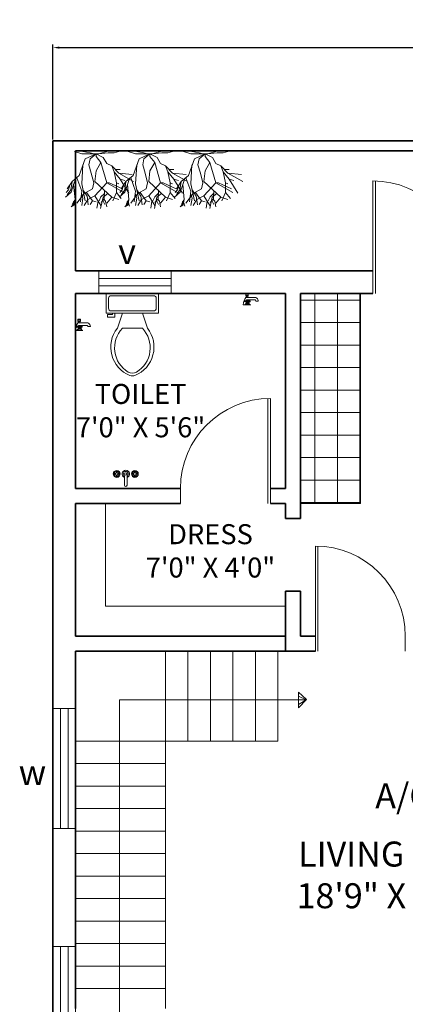
# Model space of a CAD drawing. Units: inches. Extents: x 2729 to 3178, y 5006 to 5809.
# Tile 3 of 4: x 2735 to 2889, y 5415 to 5809. Entities that reach past the tile are written whole.
import ezdxf

# ---------------------------------------------------------------- set-up
doc = ezdxf.new("R2010")
doc.units = ezdxf.units.IN
doc.layers.get('Defpoints').update_dxf_attribs({"color": 72})
for name, color, linetype, lineweight in [('A-ANNO-DIMS', 2, 'Continuous', 18), ('A-ANNO-TEXT', 7, 'Continuous', 18), ('A-AREA-IDEN', 7, 'Continuous', 25), ('A-DOOR', 4, 'Continuous', 18), ('A-FLOR-CASE', 8, 'Continuous', 18), ('A-FLOR-FIXT', 9, 'Continuous', 18), ('A-FLOR-PATT', 9, 'Continuous', 13), ('A-FLOR-STRS', 7, 'Continuous', 18), ('A-GLAZ', 4, 'Continuous', 18), ('A-WALL', 7, 'Continuous', 35), ('L-PLNT', 72, 'Continuous', 13)]:
    doc.layers.add(name, color=color, linetype=linetype, lineweight=lineweight)
doc.styles.get("Standard").update_dxf_attribs({"font": 'arial.ttf'})
doc.dimstyles.new('ISO-25', dxfattribs={"dimtxt": 2.5, "dimasz": 2.5, "dimexe": 1.25, "dimexo": 0.625, "dimtad": 1, "dimdec": 0, "dimlunit": 3, "dimtxsty": 'Standard', "dimcen": 2.5, "dimadec": 0, "dimazin": 0, "dimtfac": 1, "dimtdec": 0, "dimtmove": 0, "dimatfit": 3, "dimfxl": 1, "dimarcsym": 0})

# ---------------------------------------------------------------- blocks, each defined once
blk = doc.blocks.new('*D1')
at = {"layer": 'A-ANNO-DIMS', "color": 0, "lineweight": -2, "transparency": 16777216}
for p, q in [((2748.18, 5761.26), (2748.18, 5799.21)), ((2750.68, 5797.96), (3069.68, 5797.96)), ((3072.18, 5761.26), (3072.18, 5799.21))]:
    blk.add_line(p, q, dxfattribs=at)
at = {"layer": 'A-ANNO-DIMS', "color": 0, "transparency": 16777216}
for points in [[(2750.68, 5798.38), (2750.68, 5797.54), (2748.18, 5797.96)], [(3069.68, 5798.38), (3069.68, 5797.54), (3072.18, 5797.96)]]:
    blk.add_solid(points, dxfattribs=at)
at = {"layer": 'Defpoints', "color": 0, "transparency": 16777216}
for p in [(3072.18, 5797.96), (2748.18, 5760.64), (3072.18, 5760.64)]:
    blk.add_point(p, dxfattribs=at)
at = {"layer": 'A-ANNO-DIMS', "color": 0, "transparency": 16777216, "insert": (2910.18, 5803.61), "char_height": 2.5, "attachment_point": 5}
blk.add_mtext("{\\H4x;27'}", dxfattribs=at)
blk = doc.blocks.new('Faucet - Bathroom side')
for p, q in [((-0.625, 4.25), (0.375, 4.25)), ((-1.625, 0), (-1.375, 0)), ((-1.375, 0), (1.375, 0)), ((-0.88366, 0.25), (0.88424, 0.25)), ((0.375, 3.75), (-0.625, 3.75)), ((-0.625, 3), (3.375, 3)), ((-0.375, 1.625), (-0.625, 1.625)), ((-0.375, 1.375), (-0.625, 1.375)), ((0.48078, 0.75), (-0.47286, 0.75)), ((-0.375, 3), (-0.375, 3.5)), ((0.125, 3.5), (0.125, 3)), ((2.875, 2), (0.375, 2)), ((0.375, 1.625), (0.625, 1.625)), ((0.375, 1.375), (0.625, 1.375)), ((4.375, 1.5), (3.375, 1.5))]:
    blk.add_line(p, q)
for points in [[(-0.625, 3.75), (-0.625, 4.25)], [(-0.375, 4.5), (0.125, 4.5)], [(0.375, 4.25), (0.375, 3.75)], [(0.125, 3.5), (-0.375, 3.5)]]:
    blk.add_lwpolyline(points)
blk.add_lwpolyline([(-0.375, 1), (-0.375, 2), (0.375, 2), (0.375, 1)], close=True)
for centre in [(-0.875, 1.5), (0, 1.5), (0.875, 1.5)]:
    blk.add_circle(centre, 0.27951)
for centre, radius, start, end in [((-0.38253, 4.2575), 0.24259, 88.22243, 181.7776), ((0.13252, 4.2575), 0.24259, 358.2224, 91.77757), ((3.45929, -0.0281), 5.08436, 143.4467, 179.6834), ((-1.75, 1.375), 1.42522, 285.2551, 344.7449), ((-0.38253, 3.7424), 0.24259, 178.2224, 271.7776), ((0.13252, 3.7424), 0.24259, 268.2224, 1.777565), ((1.75, 1.375), 1.42522, 195.2551, 254.7449), ((-2.49562, -0.286), 3.38273, 9.709485, 29.48735), ((2.96867, 1.5936), 0.41699, 347.0192, 102.9808), ((2.70708, 1.4714), 1.66816, 0.9827695, 66.39737)]:
    blk.add_arc(centre, radius, start, end)
blk = doc.blocks.new('Toilet - top')
for p, q in [((9.5, -6), (9.5, -2)), ((-10, -8.5), (-8, -8.5)), ((-10, -9.5), (-10, -8.5)), ((-7, -9.5), (-10, -9.5)), ((-8, -8.5), (-8, -8)), ((-7, -8), (-7, -9.5)), ((-4, -8), (-6, -14)), ((4, -8), (6, -14)), ((4, -14), (-4, -14))]:
    blk.add_line(p, q)
blk.add_lwpolyline([(10.5, -8), (10.5, 0), (-10.5, 0), (-10.5, -8)], close=True)
for points in [[(-9.5, -2), (-9.5, -6)], [(8.5, -1), (-8.5, -1)], [(-8.5, -7), (8.5, -7)]]:
    blk.add_lwpolyline(points)
for centre, radius, start, end in [((-8.62, -1.88), 0.884, 81.8699, 188.1301), ((8.62, -1.88), 0.884, 351.8699, 98.1301), ((-8.62, -6.12), 0.884, 171.8699, 278.1301), ((8.62, -6.12), 0.884, 261.8699, 8.1301), ((3.52, -21.58), 12.17, 141.4691, 247.9714), ((4.2, -21.82), 11.33, 136.3677, 238.9468), ((-3.52, -21.58), 12.17, 292.0284, 38.5307), ((-4.2, -21.82), 11.33, 301.053, 43.6321), ((0, -27.88), 4, 245.7318, 294.2682), ((0, -29), 4, 254.8605, 285.1395)]:
    blk.add_arc(centre, radius, start, end)
blk = doc.blocks.new('Faucet - Bathroom top')
for p, q in [((-4.107, 0.125), (-4.375, 0.125)), ((-3.75, 0.4788), (-3.75, 0.75)), ((-3.5, 0.482), (-3.5, 0.75)), ((-3.1461, 0.125), (-2.875, 0.125)), ((3.143, 0.125), (2.875, 0.125)), ((3.5, 0.4788), (3.5, 0.75)), ((3.75, 0.482), (3.75, 0.75)), ((4.1039, 0.125), (4.375, 0.125)), ((-4.1039, -0.125), (-4.375, -0.125)), ((-3.75, -0.4821), (-3.75, -0.75)), ((-3.5, -0.4789), (-3.5, -0.75)), ((-3.143, -0.125), (-2.875, -0.125)), ((-0.5, -0.8639), (-0.5, -4.5)), ((0.5, -4.5), (0.5, -0.8631)), ((3.1461, -0.125), (2.875, -0.125)), ((3.5, -0.4821), (3.5, -0.75)), ((3.75, -0.4789), (3.75, -0.75)), ((4.107, -0.125), (4.375, -0.125))]:
    blk.add_line(p, q)
for centre, radius in [((-3.625, 0), 1.375), ((-4.625, 0), 0.2795), ((-3.625, 0), 0.5), ((-3.625, 1), 0.2795), ((-2.625, 0), 0.2795), ((0, 0), 0.5), ((3.625, 0), 1.375), ((2.625, 0), 0.2795), ((3.625, 0), 0.5), ((3.625, 1), 0.2795), ((4.625, 0), 0.2795), ((-3.625, -1), 0.2795), ((3.625, -1), 0.2795)]:
    blk.add_circle(centre, radius)
for centre, radius, start, end in [((-3.625, 0), 1, 105.2407, 164.2093), ((-3.625, 0), 1, 16.44125, 74.07887), ((0, 0), 1.5, 289.6514, 250.3603), ((0, 0), 1, 300.3431, 239.7554), ((3.625, 0), 1, 106.12, 164.0884), ((3.625, 0), 1, 16.23422, 73.90469), ((-3.625, 0), 1, 196.2342, 253.9047), ((-3.625, 0), 1, 286.12, 344.0884), ((3.625, 0), 1, 196.4413, 254.0789), ((3.625, 0), 1, 285.2407, 344.2093), ((0, -4.5), 0.5, 180, 0)]:
    blk.add_arc(centre, radius, start, end)
blk = doc.blocks.new('*U13')
for p, q in [((-377.952, 463.296), (-329.184, 524.256)), ((-316.7634, 502.285), (-327.6092, 559.9176)), ((-296.5958, 484.4034), (-316.7634, 502.285)), ((-286.512, 498.3226), (-307.4416, 538.0736)), ((-302.7934, 478.4344), (-270.256, 518.1854)), ((-290.3982, 464.5406), (-265.6078, 577.8246)), ((-268.7066, 458.5716), (-250.0884, 500.3038)), ((-207.264, 451.104), (-268.224, 548.64)), ((-240.792, 502.285), (-228.3968, 573.8368)), ((-182.88, 499.872), (-219.456, 512.064)), ((-182.88, 499.872), (-158.496, 536.448)), ((-129.1844, 450.6214), (-140.0302, 542.036)), ((-134.112, 487.68), (-97.536, 548.64)), ((-97.536, 426.72), (-24.384, 524.256)), ((-85.7758, 472.4908), (-73.3552, 548.005)), ((-73.152, 402.336), (-60.96, 512.064)), ((-12.9032, 555.9552), (-2.0574, 522.1732)), ((-5.1562, 486.3846), (2.5908, 542.036)), ((-3.6068, 492.3536), (14.986, 518.1854)), ((-0.508, 508.254), (22.7584, 536.067)), ((1.0414, 526.1356), (35.1536, 559.9176)), ((2.5908, 542.036), (21.209, 555.9552)), ((-463.296, 280.416), (-552.577, 423.037)), ((-329.184, 316.992), (-499.872, 414.528)), ((-426.72, 414.528), (-475.488, 475.488)), ((-377.952, 463.296), (-451.104, 487.68)), ((-426.72, 414.528), (-390.144, 499.872)), ((-426.72, 316.992), (-426.72, 414.528)), ((-207.264, 304.8), (-377.952, 463.296)), ((-338.455, 424.7896), (-290.3982, 464.5406)), ((-329.184, 316.992), (-207.264, 451.104)), ((-305.8922, 396.9512), (-302.7934, 478.4344)), ((-304.3428, 426.7708), (-268.7066, 458.5716)), ((-207.264, 451.104), (-134.112, 487.68)), ((-121.92, 414.528), (-182.88, 499.872)), ((-182.88, 377.952), (-97.536, 426.72)), ((-85.7758, 389.001), (-129.1844, 452.6026)), ((-73.152, 329.184), (-109.728, 499.872)), ((-70.2564, 426.7708), (-85.7758, 472.4908)), ((-24.384, 268.224), (-73.152, 402.336)), ((8.7884, 335.3562), (-5.1562, 486.3846)), ((8.7884, 335.3562), (33.6042, 412.8516)), ((33.6042, 412.8516), (92.5068, 464.5406)), ((36.576, 390.144), (73.152, 438.912)), ((60.96, 390.144), (85.344, 414.528)), ((-451.104, 219.456), (-601.0402, 303.8094)), ((-353.568, 316.992), (-487.68, 377.952)), ((-426.72, 316.992), (-451.104, 329.184)), ((-402.336, 207.264), (-426.72, 316.992)), ((-329.184, 316.992), (-353.568, 316.992)), ((-268.224, 109.728), (-329.184, 316.992)), ((-219.456, 195.072), (-207.264, 304.8)), ((-195.072, 316.992), (-182.88, 377.952)), ((-170.688, 219.456), (-195.072, 316.992)), ((-85.344, 134.112), (-73.152, 329.184)), ((-48.768, 243.84), (24.384, 304.8)), ((-12.192, 274.32), (8.7884, 335.3562)), ((24.384, 304.8), (36.576, 390.144)), ((24.384, 304.8), (73.152, 377.952)), ((48.768, 341.376), (60.96, 390.144)), ((-451.104, 219.456), (-587.4512, 234.2388)), ((-463.296, 280.416), (-512.064, 292.608)), ((-402.336, 207.264), (-463.296, 280.416)), ((-377.952, 146.304), (-451.104, 219.456)), ((-377.952, 146.304), (-402.336, 207.264)), ((-146.304, 134.112), (-170.688, 219.456)), ((-109.728, 73.152), (-48.768, 243.84)), ((-414.528, 182.88), (-463.296, 182.88)), ((-329.184, 121.92), (-377.952, 146.304)), ((-292.608, 60.96), (-329.184, 121.92)), ((-268.224, 109.728), (-219.456, 195.072)), ((-219.456, 48.768), (-268.224, 109.728)), ((-158.496, 73.152), (-146.304, 134.112)), ((-402.336, 12.192), (-451.104, 0)), ((-341.376, 12.192), (-402.336, 12.192)), ((-243.84, 24.384), (-341.376, 12.192)), ((-243.84, 24.384), (-329.184, 0)), ((-219.456, 24.384), (-292.608, 60.96)), ((-243.84, 24.384), (-195.072, 24.384)), ((-219.456, 24.384), (-109.728, 73.152)), ((-219.456, 24.384), (-158.496, 73.152)), ((-219.456, 24.384), (-219.456, 48.768)), ((-219.456, 24.384), (-73.152, 24.384)), ((-195.072, 24.384), (-158.496, 12.192)), ((-158.496, 12.192), (-85.344, 0)), ((-73.152, 24.384), (0, 0))]:
    blk.add_line(p, q)
blk = doc.blocks.new('WIN-48IN')
for p, q in [((48, 9), (0, 9)), ((0, 9), (0, 0)), ((48, 0), (48, 9)), ((48, 6), (0, 6)), ((0, 3), (48, 3)), ((0, 0), (48, 0))]:
    blk.add_line(p, q)
blk = doc.blocks.new('DOOR-36IN-JAMB6')
for p, q in [((0, 6), (0, 42)), ((1, 6), (1, 42)), ((0, 6), (0, 0)), ((1, 6), (1, 0)), ((36, 0), (36, 6))]:
    blk.add_line(p, q)
blk.add_arc((0, 6), 36, 0, 90)
blk = doc.blocks.new('VENT-29IN')
for p, q in [((29, 9), (0, 9)), ((0, 9), (0, 0)), ((29, 0), (29, 9)), ((29, 6), (0, 6)), ((0, 3), (29, 3)), ((0, 0), (29, 0))]:
    blk.add_line(p, q)

msp = doc.modelspace()

# ---------------------------------------------------------------- hatches: boundary and pattern name
at = {"layer": 'A-FLOR-PATT'}
h = msp.add_hatch(dxfattribs=at)
h.set_pattern_fill('ANSI37', color=256, scale=2.834646, angle=-45, style=0)
h.paths.add_polyline_path([(2847.18, 5615.64), (2871.18, 5615.64), (2871.18, 5699.64), (2847.18, 5699.64)])

# ---------------------------------------------------------------- linework, layer by layer
at = {"layer": 'A-DOOR'}
for p, q in [((2876.18, 5699.64), (2876.18, 5744.64)), ((2877.18, 5699.64), (2877.18, 5744.64)), ((2876.18, 5699.64), (2876.18, 5708.64))]:
    msp.add_line(p, q, dxfattribs=at)
msp.add_arc((2876.18, 5708.64), 36, 0, 90, dxfattribs=at)
at = {"layer": 'A-FLOR-CASE'}
for p, q in [((2871.18, 5615.64), (2871.18, 5699.64)), ((2757.18, 5615.64), (2769.18, 5615.64)), ((2769.18, 5615.64), (2769.18, 5574.64)), ((2847.18, 5615.64), (2871.18, 5615.64)), ((2841.18, 5574.64), (2769.18, 5574.64)), ((2841.18, 5562.64), (2841.18, 5574.64))]:
    msp.add_line(p, q, dxfattribs=at)
at = {"layer": 'A-FLOR-STRS'}
for p, q in [((2793.18, 5419.64), (2793.18, 5556.64)), ((2802.18, 5520.64), (2802.18, 5556.64)), ((2811.18, 5520.64), (2811.18, 5556.64)), ((2820.18, 5520.64), (2820.18, 5556.64)), ((2829.18, 5520.64), (2829.18, 5556.64)), ((2838.18, 5520.64), (2838.18, 5556.64)), ((2846.48, 5537.18), (2846.48, 5540.14)), ((2846.48, 5540.14), (2846.48, 5533.92)), ((2849.58, 5537.21), (2846.48, 5540.14)), ((2846.48, 5540.14), (2846.48, 5537.18)), ((2774.75, 5385.44), (2774.75, 5537.18)), ((2774.75, 5537.18), (2846.48, 5537.18)), ((2849.55, 5537.18), (2846.48, 5538.66)), ((2846.48, 5538.66), (2849.55, 5537.18)), ((2846.48, 5533.92), (2849.58, 5537.21)), ((2846.48, 5537.18), (2849.55, 5537.18)), ((2849.55, 5537.18), (2846.48, 5535.3)), ((2757.18, 5520.64), (2838.18, 5520.64)), ((2757.18, 5511.64), (2793.18, 5511.64)), ((2757.18, 5502.64), (2793.18, 5502.64)), ((2757.18, 5493.64), (2793.18, 5493.64)), ((2757.18, 5484.64), (2793.18, 5484.64)), ((2757.18, 5475.64), (2793.18, 5475.64)), ((2757.18, 5466.64), (2793.18, 5466.64)), ((2757.18, 5457.64), (2793.18, 5457.64)), ((2757.18, 5448.64), (2793.18, 5448.64)), ((2757.18, 5439.64), (2793.18, 5439.64)), ((2757.18, 5430.64), (2793.18, 5430.64)), ((2757.18, 5421.64), (2793.18, 5421.64)), ((2793.18, 5419.64), (2793.18, 5413.64))]:
    msp.add_line(p, q, dxfattribs=at)
at = {"layer": 'A-WALL'}
for p, q in [((2748.18, 5760.64), (3072.18, 5760.64)), ((2748.18, 5112.64), (2748.18, 5760.64)), ((2757.18, 5756.64), (3063.18, 5756.64)), ((2757.18, 5708.64), (2757.18, 5756.64)), ((2757.18, 5708.64), (2876.18, 5708.64)), ((2757.18, 5699.64), (2841.18, 5699.64)), ((2757.18, 5621.64), (2757.18, 5699.64)), ((2841.18, 5621.64), (2841.18, 5699.64)), ((2847.18, 5699.64), (2876.18, 5699.64)), ((2847.18, 5609.64), (2847.18, 5699.64)), ((2871.18, 5699.64), (2876.18, 5699.64)), ((2757.18, 5621.64), (2799.18, 5621.64)), ((2841.18, 5621.64), (2835.18, 5621.64)), ((2835.18, 5621.64), (2841.18, 5621.64)), ((2757.18, 5615.64), (2799.18, 5615.64)), ((2757.18, 5562.64), (2757.18, 5615.64)), ((2835.18, 5615.64), (2841.18, 5615.64)), ((2841.18, 5615.64), (2841.18, 5609.64)), ((2841.18, 5609.64), (2841.18, 5615.64)), ((2841.18, 5609.64), (2847.18, 5609.64)), ((2841.18, 5562.64), (2841.18, 5580.64)), ((2847.18, 5580.64), (2841.18, 5580.64)), ((2847.18, 5562.64), (2847.18, 5580.64)), ((2757.18, 5562.64), (2841.18, 5562.64)), ((2841.18, 5562.64), (2841.18, 5556.64)), ((2847.18, 5562.64), (2853.18, 5562.64)), ((2847.18, 5562.64), (2853.18, 5562.64)), ((2847.18, 5562.64), (2853.18, 5562.64)), ((2757.18, 5556.64), (2853.18, 5556.64)), ((2757.18, 5419.64), (2757.18, 5556.64)), ((2757.18, 5419.64), (2757.18, 5413.64))]:
    msp.add_line(p, q, dxfattribs=at)

# ---------------------------------------------------------------- block references
at = {"layer": 'A-DOOR', "extrusion": (0, 0, -1), "zscale": -1}
msp.add_blockref('DOOR-36IN-JAMB6', (-2835.18, 5615.64), dxfattribs=at)
at = {"layer": 'A-DOOR'}
msp.add_blockref('DOOR-36IN-JAMB6', (2853.18, 5556.64), dxfattribs=at)
at = {"layer": 'A-FLOR-FIXT'}
for name, p in [('Toilet - top', (2779.96, 5699.71)), ('Faucet - Bathroom side', (2825.98, 5695.05)), ('Faucet - Bathroom side', (2758.78, 5684.87)), ('Faucet - Bathroom top', (2777.32, 5627.46))]:
    msp.add_blockref(name, p, dxfattribs=at)
at = {"layer": 'A-GLAZ'}
msp.add_blockref('VENT-29IN', (2766.5, 5699.64), dxfattribs=at)
for p, rotation in [((2757.26, 5485.69), 90.00000000000003), ((2757.26, 5390.54), 89.99999999999935)]:
    msp.add_blockref('WIN-48IN', p, dxfattribs=dict(at, rotation=rotation))
at = {"layer": 'L-PLNT', "xscale": 0.0393700787401575, "yscale": 0.0393700787401575, "zscale": 0.0393700787401575, "rotation": 180}
for p in [(2756.8, 5756.38), (2778.32, 5756.38), (2800.45, 5756.38)]:
    msp.add_blockref('*U13', p, dxfattribs=at)

# ---------------------------------------------------------------- texts
at = {"layer": 'A-ANNO-TEXT', "char_height": 10, "attachment_point": 1}
for s, width, insert in [('v', 9.2139, (2774.29, 5721.46)), ('w', 11.1436, (2734.5, 5513.08)), ('\\pxqc;A/O', 28.8912, (2874.59, 5503.75))]:
    msp.add_mtext_dynamic_manual_height_columns(s, width=width, gutter_width=12.5, heights=[0], dxfattribs=dict(at, insert=insert))
at = {"layer": 'A-AREA-IDEN', "attachment_point": 1}
for s, width, insert, char_height in [('\\pxqc;TOILET\\P7\'0" X 5\'6"', 56.6074, (2754.93, 5663.46), 8), ('\\pxqc;DRESS\\P7\'0" X 4\'0"', 68.6474, (2776.89, 5607.38), 8), ('\\pxqc;LIVING HALL\\P18\'9" X 11\'5"', 114.8323, (2828.17, 5480.46), 10)]:
    msp.add_mtext_dynamic_manual_height_columns(s, width=width, gutter_width=12.5, heights=[0], dxfattribs=dict(at, insert=insert, char_height=char_height))

# ---------------------------------------------------------------- dimensions: what is measured, and where the dimension line sits
at = {"layer": 'A-ANNO-DIMS'}
dim = msp.add_linear_dim(base=(3072.18, 5797.96), p1=(2748.18, 5760.64), p2=(3072.18, 5760.64), text="{\\H4x;27'}", dimstyle='ISO-25', override={"dimclrd": 0, "dimclre": 0, "dimclrt": 0}, dxfattribs=at)
dim.commit()
dim.dimension.update_dxf_attribs({"geometry": '*D1', "text_midpoint": (2910.18, 5803.61)})

doc.saveas('drawing.dxf')
